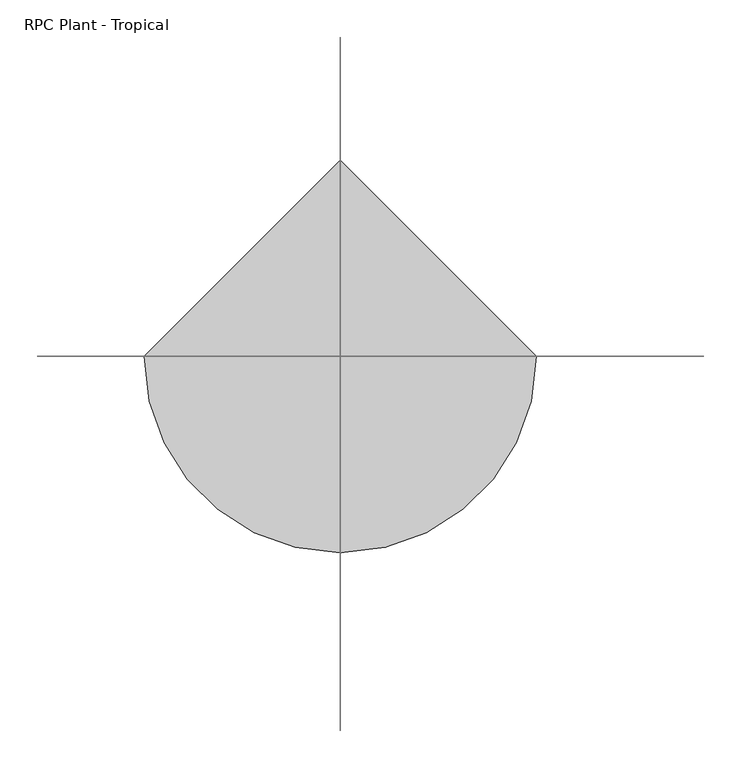
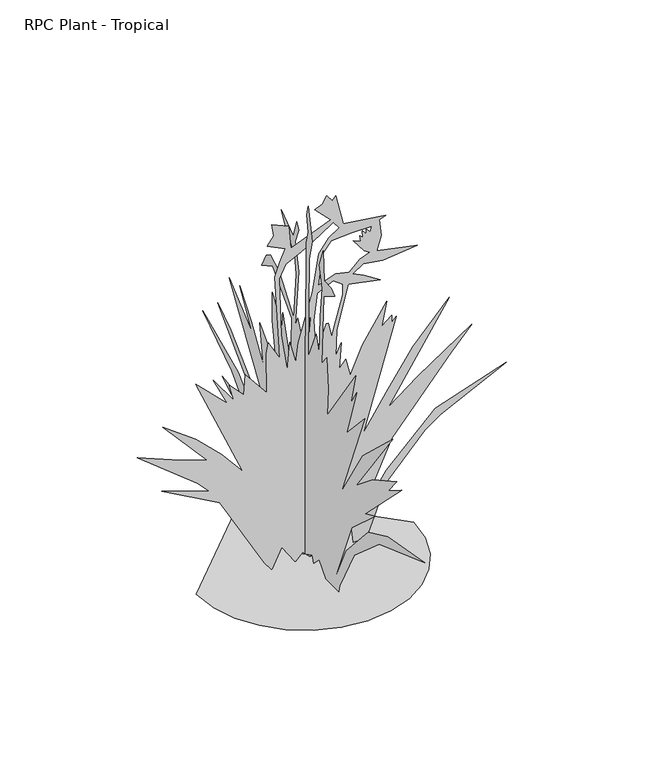
"""IFC4 building model written with IfcOpenShell, lengths in millimetres: geographic element geometry, RPC Plant - Tropical."""

from ifc_helpers import new_model, si_unit, origin, place, context, project, spatial, triangles, source, transform, mapped, element, save


def rpc_plant_tropical_55f6ff97(model_context):
    return source(origin(), model_context, "Body", "Tessellation", [
        triangles([(-264.3380075, 0.0, 0.0272524), (-257.3504617, -60.5688865, 0.0272524), (-237.4475159, -116.1916269, 0.0272524), (-206.2245489, -165.274632, 0.0272524), (-165.274632, -206.2245489, 0.0272524), (-116.1916269, -237.4475159, 0.0272524), (-60.5688865, -257.3504617, 0.0272524), (1.16e-05, -264.3380075, 0.0272524), (60.5688865, -257.3504617, 0.0272524), (116.1916269, -237.4475159, 0.0272524), (165.274632, -206.2245489, 0.0272524), (206.2245489, -165.274632, 0.0272524), (237.4475159, -116.1916269, 0.0272524), (257.3504617, -60.5688865, 0.0272524), (264.3380075, 2.31e-05, 0.0272524), (-3.47e-05, 264.3380075, 0.0272524), (-5.2e-06, -141.3706678, 0.0), (-2.8e-06, -89.4159448, 0.054498), (-3.14e-05, -59.9343958, 33.2735186), (-3.1e-05, -36.3827356, 9.846953), (-3.03e-05, -30.3380374, 26.1345898), (2.2e-06, 22.1351019, 0.0353721), (-2.75e-05, 35.0893666, 22.475361), (-2.7e-05, 50.4325003, 13.9824575), (-2.41e-05, 71.8028075, 80.7852761), (5.2e-06, 91.613049, 0.0211753), (-2.36e-05, 109.0153662, 40.8424698), (-2.42e-05, 112.8357816, 15.9965016), (-1.83e-05, 164.4437961, 134.5614359), (-1.5e-05, 201.3025201, 190.8125718), (-8.6e-06, 314.8967674, 236.0083596), (-6.4e-06, 348.2342674, 257.8737037), (-8.8e-06, 301.5160253, 250.5209003), (-1.18e-05, 246.732487, 231.9590791), (-7.1e-06, 309.0598417, 295.0364789), (8e-07, 430.3017509, 376.6543714), (-7.9e-06, 280.4721063, 309.3519387), (-1.58e-05, 174.5674878, 204.3200503), (-9.8e-06, 240.1660818, 307.4037292), (-3e-07, 367.670363, 434.9626582), (-3.8e-06, 312.5929836, 399.2629114), (-1.14e-05, 210.1351387, 300.3374635), (-1.65e-05, 148.1844779, 220.8381918), (-1.17e-05, 187.1702069, 323.3016323), (3e-07, 320.1596366, 527.8276657), (-6.4e-06, 222.976615, 445.7627257), (-1.5e-06, 274.807899, 534.3072121), (-5.5e-06, 226.7299833, 472.9153562), (-1.02e-05, 175.4651256, 391.7724529), (-6.5e-06, 190.5821898, 491.1144633), (-1.2e-05, 119.3145649, 415.5265626), (-7.8e-06, 137.4532288, 529.6031387), (-5.6e-06, 138.7511692, 601.2540341), (-9.5e-06, 94.9513718, 536.1969586), (-8.4e-06, 93.3989229, 575.3383922), (-1.32e-05, 59.5732078, 463.4487828), (-9.8e-06, 56.2066891, 583.9388483), (-3.7e-06, 136.0049161, 669.1432405), (-2.4e-06, 181.9436545, 644.4467829), (-2.1e-06, 163.9243692, 680.6875214), (-2.5e-06, 147.0399529, 691.5511024), (-4.8e-06, 108.1804607, 671.9067347), (-1e-05, 48.046931, 590.4565101), (-6.9e-06, 36.8709235, 709.0745968), (-5.3e-06, 43.8627887, 753.7100264), (-2e-06, 83.7514831, 804.4440662), (-3e-07, 99.8779606, 836.6538008), (-3.7e-06, 49.136086, 799.8898384), (-2.9e-06, 35.0893666, 845.2923723), (-3.8e-06, 26.4505657, 828.0152292), (-4.3e-06, 41.5678933, 791.3020632), (-7e-06, 26.8495989, 721.233593), (-1.07e-05, 41.5678933, 575.3383922), (-1.05e-05, 30.7698379, 599.0950453), (-1.29e-05, 9.1735731, 551.5843188), (-1.27e-05, -4.2437592, 577.167205), (-5.7e-06, -6.2811965, 815.731822), (-5.1e-06, -13.569935, 847.4513248), (-3.6e-06, -6.9461944, 887.7586756), (-3.1e-06, -14.582304, 914.4007267), (-6.2e-06, -30.3001922, 833.2324253), (-7.2e-06, -17.1413308, 780.7407166), (-1.46e-05, -14.582304, 527.8276657), (-1.38e-05, -46.9765748, 605.5745916), (-1.57e-05, -59.9343958, 560.222854), (-1.28e-05, -63.7807226, 662.0591526), (-1.1e-05, -73.6229771, 738.5157503), (-8.8e-06, -59.9343958, 791.3020632), (-8.5e-06, -68.5729447, 815.05868), (-8.2e-06, -77.2114935, 838.812826), (-1.06e-05, -81.5307611, 763.227396), (-1.2e-05, -110.9300204, 761.8202871), (-1.3e-05, -126.4778813, 751.5510738), (-1.23e-05, -100.3333834, 735.2899298), (-1.17e-05, -79.708316, 722.0590513), (-1.66e-05, -70.7324513, 545.1047725), (-1.68e-05, -92.3897821, 572.3361045), (-1.94e-05, -98.8076044, 495.4324774), (-2.12e-05, -94.4883277, 426.3240867), (-2.14e-05, -213.2677237, 599.0950453), (-2.3e-05, -193.8311193, 517.0301053), (-2.28e-05, -217.5869913, 558.0613217), (-2.48e-05, -176.5542669, 430.6446442), (-2.57e-05, -252.1411685, 512.7095841), (-2.87e-05, -152.798395, 264.3532501), (-2.83e-05, -244.4081376, 413.0424482), (-3.04e-05, -369.3264393, 531.0712541), (-2.98e-05, -215.4274755, 318.343541), (-3.13e-05, -285.475907, 376.1107999), (-3.42e-05, -387.58906, 431.8587779), (-3.39e-05, -351.4829427, 387.4518954), (-3.53e-05, -406.9616784, 422.1127885), (-3.3e-05, -254.1018046, 269.3443517), (-3.43e-05, -295.3336628, 288.109885), (-3.26e-05, -197.6014924, 198.8161167), (-3.48e-05, -118.2442087, 7.3579794), (-3.37e-05, -173.2017281, 125.4509545), (-3.48e-05, -266.8272088, 229.6761334), (-3.73e-05, -347.9879162, 267.302198), (-4.35e-05, -504.8177693, 294.5894314), (-3.69e-05, -312.1281501, 226.3418711), (-3.5e-05, -207.3218293, 133.5593986), (-3.57e-05, -146.3193573, 18.1561127), (117.3305654, 2.31e-05, 0.0405123), (110.3389591, 2.08e-05, 74.4091073), (78.0842327, 2.54e-05, 21.0145808), (55.6151237, 2.49e-05, 46.2313396), (12.5873108, 2.89e-05, 0.0122306), (-5.1707583, 2.92e-05, 18.1490262), (-24.1045425, 3.09e-05, 0.0037426), (-56.6857342, 2.97e-05, 48.3908508), (-81.2114855, 3.28e-05, 0.0181663), (-98.986418, 3.3e-05, 24.1438615), (-207.7917316, 2.63e-05, 216.6390658), (-348.2342674, 2.78e-05, 294.5894314), (-233.774666, 2.51e-05, 255.7146967), (-261.6024369, 2.45e-05, 285.2828592), (-408.7041229, 2.4e-05, 402.5700133), (-324.6782925, 2.24e-05, 368.0386909), (-238.0939517, 2.05e-05, 335.6206115), (-346.0752786, 1.79e-05, 458.719275), (-266.2303157, 1.79e-05, 400.2179767), (-203.8244956, 1.88e-05, 339.715129), (-151.7089902, 2.02e-05, 277.3123428), (-266.1693456, 9.5e-06, 540.784215), (-189.3886398, 1.06e-05, 466.0141786), (-222.976615, 7.9e-06, 536.4662009), (-173.7341084, 9.8e-06, 467.1774796), (-184.1031521, 7.7e-06, 510.5505589), (-149.5492202, 8.4e-06, 473.8373929), (-145.2299525, 5.2e-06, 523.5096517), (-93.3989229, 6.8e-06, 458.719275), (-94.0984351, 9e-07, 559.4354384), (-89.0799006, -9e-07, 586.138496), (-61.0044976, 8e-07, 536.4662009), (-64.4230889, -1.9e-06, 583.7153154), (-73.364658, -1.14e-05, 749.2980864), (-61.7167134, -1.39e-05, 783.3111992), (-47.9079951, -1.63e-05, 813.4864649), (-91.2394163, -1.57e-05, 834.4947756), (-76.5455003, -1.76e-05, 856.3946743), (-80.4413563, -1.92e-05, 886.3260595), (-39.8899707, -2e-05, 869.0464457), (-35.0893666, -1.67e-05, 810.7381588), (62.093907, -2.33e-05, 849.6128935), (23.2207756, -2.39e-05, 888.4850847), (42.4165107, -2.52e-05, 896.5013105), (53.4556125, -2.67e-05, 914.4007267), (66.1944834, -2.63e-05, 896.8848627), (74.7598808, -2.72e-05, 906.7806976), (93.6785752, -2.34e-05, 828.1498867), (196.1872255, -2.7e-05, 813.9157265), (180.8732984, -2.6e-05, 808.5791336), (185.7325766, -2.37e-05, 766.8723043), (174.394515, -2.11e-05, 730.8322803), (273.7385602, -2.41e-05, 709.2371595), (189.3833167, -2e-05, 700.9592491), (142.0676456, -1.83e-05, 708.1576469), (116.0844387, -1.62e-05, 691.9600891), (142.8525086, -1.66e-05, 679.102589), (183.0330503, -1.68e-05, 653.0853544), (105.3178811, -1.44e-05, 669.0848139), (77.0491851, -6.7e-06, 560.5047772), (75.051728, -2.7e-06, 495.4324774), (87.9216592, -5e-06, 524.393573), (83.6900225, -9e-07, 458.719275), (98.8076044, -2.7e-06, 478.1553706), (109.6056554, -5e-07, 432.803633), (138.9439536, -5.8e-06, 499.7708027), (199.0078928, -1.39e-05, 592.0084502), (187.352336, -9.8e-06, 532.1482232), (211.1082079, -1.2e-05, 551.5843188), (211.1082079, -1.1e-05, 534.3072121), (221.9062589, -1.21e-05, 545.1047725), (142.0000807, 7.6e-06, 272.9918035), (197.3987977, 1e-07, 358.912431), (262.4025334, -8.4e-06, 452.8214155), (351.4829427, -1.8e-05, 549.4227502), (202.4694002, 2.3e-06, 318.343541), (273.8909673, -4.1e-06, 372.7275035), (405.4757589, -1.51e-05, 460.8783002), (355.6612487, -9.6e-06, 405.7856601), (211.5270596, 6.8e-06, 235.3906284), (131.6828507, 2.08e-05, 59.5396797), (197.4798247, 1.2e-05, 158.3333043), (317.0659301, -2e-07, 275.0161712), (489.6996878, -1.12e-05, 333.4616226), (330.1571005, 5e-07, 255.2422691), (291.8284444, 3.8e-06, 227.7759587), (199.2240496, 1.38e-05, 127.0808696), (148.478864, 2.13e-05, 0.0507429), (114.3788288, -2.24e-05, 797.4488537), (63.6714996, -2.01e-05, 794.7361559), (42.3199913, -1.75e-05, 767.5631779), (31.8592449, -1.25e-05, 691.9600891), (74.6966352, -1.53e-05, 706.3237473), (107.4461487, -1.62e-05, 698.437092), (132.807564, -1.88e-05, 722.7067589), (157.1176626, -2.05e-05, 732.9912329), (143.9299774, -2.04e-05, 741.276701), (117.5705943, -2.13e-05, 776.2906248), (135.9680906, -2.16e-05, 768.3049204), (133.7021497, -2.24e-05, 783.2401279), (140.693002, -2.24e-05, 777.0983517), (139.840574, -2.33e-05, 793.4610884), (148.478864, -2.3e-05, 782.6634916), (148.8047525, -2.38e-05, 795.162874), (158.4753014, -2.36e-05, 785.4854851), (162.2614257, -2.45e-05, 797.6698431), (36.4967821, -2.03e-05, 819.0008085), (-10.5179706, -1.66e-05, 790.7762959), (-46.6034508, -1.4e-05, 773.6338102), (-62.8378705, -1.14e-05, 741.9143074), (-57.6440741, -2.8e-06, 594.8100597), (-43.7276589, 2.2e-06, 499.7530349), (-37.2488755, -2.2e-06, 568.8613893), (-22.1313685, 5e-07, 512.7095841), (-15.8925131, -2.6e-06, 559.8647), (18.0916476, -1.1e-05, 677.0451565), (33.6138798, -1.74e-05, 772.2038103), (57.6697312, -2.04e-05, 805.3914648), (83.6900225, -2.25e-05, 821.5356829), (68.5729447, -2.3e-05, 840.9743219), (30.2087529, -1.13e-05, 671.65784), (21.8014718, -6.9e-06, 605.0462809), (25.6817059, -2.5e-06, 528.0867342), (30.8554363, -2.8e-06, 528.7344418), (51.5501011, -7.1e-06, 586.290885), (56.0771503, -7.3e-06, 585.6457209), (65.1309854, -5.4e-06, 548.1349654), (69.6580301, -6.8e-06, 568.1831966), (91.6460685, -1.24e-05, 645.7879074), (91.6460685, -1.4e-05, 672.9507116), (68.3644091, -1.4e-05, 690.4106197), (6.9271952, -5.7e-06, 595.3460009), (10.8074288, -4.5e-06, 573.3571904), (13.394269, -6.1e-06, 597.9317079), (15.3343985, -7.9e-06, 627.035055)], [[15, 16, 1], [14, 15, 1], [14, 1, 2], [13, 14, 2], [13, 2, 3], [13, 3, 4], [12, 13, 4], [11, 12, 4], [11, 4, 5], [11, 5, 6], [11, 6, 7], [11, 7, 8], [11, 8, 9], [11, 9, 10], [46, 47, 48], [119, 120, 121], [35, 36, 37], [106, 107, 108], [39, 40, 41], [39, 41, 42], [101, 102, 103], [111, 112, 113], [105, 106, 108], [44, 45, 46], [113, 114, 115], [54, 55, 56], [103, 104, 105], [99, 100, 101], [109, 110, 111], [89, 90, 91], [118, 119, 121], [31, 32, 33], [46, 48, 49], [44, 46, 49], [79, 80, 81], [78, 79, 81], [66, 67, 68], [27, 28, 29], [52, 53, 54], [88, 89, 91], [87, 88, 91], [49, 50, 51], [58, 59, 60], [99, 101, 103], [25, 26, 27], [83, 84, 85], [109, 111, 113], [108, 109, 113], [96, 97, 98], [68, 69, 70], [68, 70, 71], [38, 39, 42], [38, 42, 43], [65, 66, 68], [65, 68, 71], [65, 71, 72], [64, 65, 72], [64, 72, 73], [63, 64, 73], [118, 121, 122], [117, 118, 122], [117, 122, 123], [116, 117, 123], [73, 74, 75], [116, 123, 17], [116, 17, 18], [58, 60, 61], [58, 61, 62], [57, 58, 62], [57, 62, 63], [77, 78, 81], [77, 81, 82], [76, 77, 82], [76, 82, 83], [75, 76, 83], [92, 93, 94], [19, 20, 21], [30, 31, 33], [30, 33, 34], [91, 92, 94], [87, 91, 94], [87, 94, 95], [86, 87, 95], [86, 95, 96], [85, 86, 96], [34, 35, 37], [34, 37, 38], [30, 34, 38], [25, 27, 29], [57, 63, 73], [56, 57, 73], [56, 73, 75], [56, 75, 83], [23, 24, 25], [99, 103, 105], [29, 30, 38], [105, 108, 113], [105, 113, 115], [51, 52, 54], [51, 54, 56], [83, 85, 96], [21, 22, 23], [83, 96, 98], [83, 98, 99], [56, 83, 99], [29, 38, 43], [25, 29, 43], [115, 116, 18], [115, 18, 19], [105, 115, 19], [21, 23, 25], [44, 49, 51], [43, 44, 51], [56, 99, 105], [51, 56, 105], [43, 51, 105], [43, 105, 19], [25, 43, 19], [21, 25, 19], [248, 124, 125], [241, 229, 212], [206, 207, 208], [197, 198, 199], [146, 147, 148], [134, 135, 136], [196, 197, 199], [241, 212, 213], [255, 237, 238], [140, 141, 142], [200, 201, 202], [137, 138, 139], [255, 238, 239], [258, 255, 239], [175, 176, 177], [184, 185, 186], [235, 236, 237], [180, 181, 182], [189, 190, 191], [144, 145, 146], [140, 142, 143], [247, 248, 125], [171, 172, 173], [200, 202, 203], [199, 200, 203], [193, 194, 195], [237, 255, 256], [220, 221, 222], [148, 149, 150], [137, 139, 140], [224, 225, 226], [229, 241, 242], [195, 196, 199], [222, 223, 224], [153, 154, 155], [179, 180, 182], [150, 151, 152], [226, 227, 228], [191, 192, 193], [186, 187, 188], [169, 170, 171], [175, 177, 178], [152, 153, 155], [195, 199, 203], [161, 162, 163], [240, 241, 213], [240, 213, 214], [165, 166, 167], [167, 168, 169], [165, 167, 169], [165, 169, 171], [191, 193, 195], [189, 191, 195], [188, 189, 195], [239, 240, 214], [239, 214, 215], [125, 126, 127], [124, 248, 249], [124, 249, 250], [161, 163, 164], [160, 161, 164], [159, 160, 164], [131, 132, 133], [144, 146, 148], [129, 130, 131], [131, 133, 134], [206, 208, 209], [205, 206, 209], [205, 209, 210], [204, 205, 210], [204, 210, 211], [204, 211, 124], [204, 124, 250], [246, 247, 125], [195, 203, 204], [144, 148, 150], [144, 150, 152], [158, 159, 164], [127, 128, 129], [246, 125, 127], [246, 127, 129], [246, 129, 131], [136, 137, 140], [136, 140, 143], [136, 143, 144], [134, 136, 144], [131, 134, 144], [220, 222, 224], [220, 224, 226], [220, 226, 228], [219, 220, 228], [131, 144, 152], [258, 239, 215], [174, 175, 178], [186, 188, 195], [215, 216, 217], [131, 152, 155], [157, 158, 164], [217, 218, 219], [186, 195, 204], [219, 228, 229], [245, 246, 131], [245, 131, 215], [244, 245, 215], [254, 244, 215], [254, 215, 217], [253, 254, 217], [252, 253, 217], [257, 258, 215], [184, 186, 204], [184, 204, 250], [183, 184, 250], [183, 250, 251], [182, 183, 251], [182, 251, 252], [182, 252, 217], [179, 182, 217], [179, 217, 219], [178, 179, 219], [174, 178, 219], [174, 219, 229], [173, 174, 229], [171, 173, 229], [171, 229, 242], [165, 171, 242], [165, 242, 243], [165, 243, 230], [164, 165, 230], [164, 230, 231], [164, 231, 232], [157, 164, 232], [157, 232, 233], [156, 157, 233], [156, 233, 234], [156, 234, 235], [155, 156, 235], [131, 155, 235], [131, 235, 237], [131, 237, 256], [215, 131, 256], [257, 215, 256]], closed=False),
    ])


if __name__ == "__main__":
    model = new_model("IFC4")
    model_context = context("Model", 3, world=origin())
    ifc_project = project(units=[si_unit("LENGTHUNIT", "METRE", prefix="MILLI")], contexts=[model_context])
    site = spatial("IfcSite", under=ifc_project)
    building = spatial("IfcBuilding", under=site)
    placement = place(None, origin())
    rpc_plant_tropical_shape = rpc_plant_tropical_55f6ff97(model_context)
    element("IfcGeographicElement", 1, ObjectType="RPC Plant - Tropical", at=placement, inside=building, context=model_context, shape_type="MappedRepresentation", body=[
        mapped(rpc_plant_tropical_shape, transform((0.0, 0.0, 0.0), x_axis=(1.0, 0.0, 0.0), y_axis=(0.0, 1.0, 0.0), z_axis=(0.0, 0.0, 1.0))),
    ])
    save(model, "model.ifc")

# Revit data of these elements
# Type "RPC Plant - Tropical"
#   built-in parameter 1005198 = "{2, 15},{39, RPC-16-FWM5-GM7X-C67P-4000-ST1L-LVER-AU},{1, 0},{1, 0},{2, 13},{1, 8},{5, Color},{1, 0},{1, 0},{3, 0.8},{3, 0.8},{3, 0.8},{1, 8},{7, BBoxMin},{1, 0},{1, 0},{1, 0},{1, 0},{1, 0},{1, 8},{7, BBoxMax},{1, 0},{1, 0},{1, 0},{1, 0},{1, 0},{2, 11},{9, RPCTypeId},{1, 0},{1, 0},{39, RPC-16-FWM5-GM7X-C67P-4000-ST1L-LVER-AU},{1, 6},{14, RPCPlantHeight},{1, 0},{1, 0},{1, 3},{2, 11},{7, keyword},{1, 0},{1, 0},{35, :RPCs:Shrubs [General]:Geometry:RPC},{2, 11},{8, category},{1, 0},{1, 0},{16, Shrubs [General]},{2, 11},{12, LocalizedUID},{1, 0},{1, 0},{10, Crane Lily},{2, 14},{6, Height},{1, 0},{1, 0},{1, 3},{1, 2},{16, Cast Reflections},{1, 0},{1, 0},{1, 0},{1, 2},{12, Cast Shadows},{1, 0},{1, 0},{1, 1},{1, 2},{9, Lock View},{1, 0},{1, 0},{1, 0},{1, 4},{5, ViewC},{1, 0},{1, 0},{1, 0},{21, assetlibrary_base.fbx},{1, 5},"
#   built-in parameter 1005195 = "RPC-16-FWM5-GM7X-C67P-4000-ST1L-LVER-AU"
#   Assembly Code = "G2050500"
#   Height = 3' - 0"
#   Default Elevation = 0
